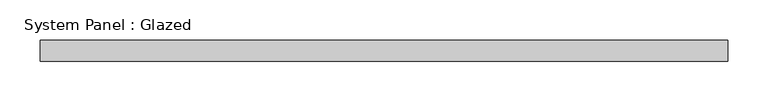
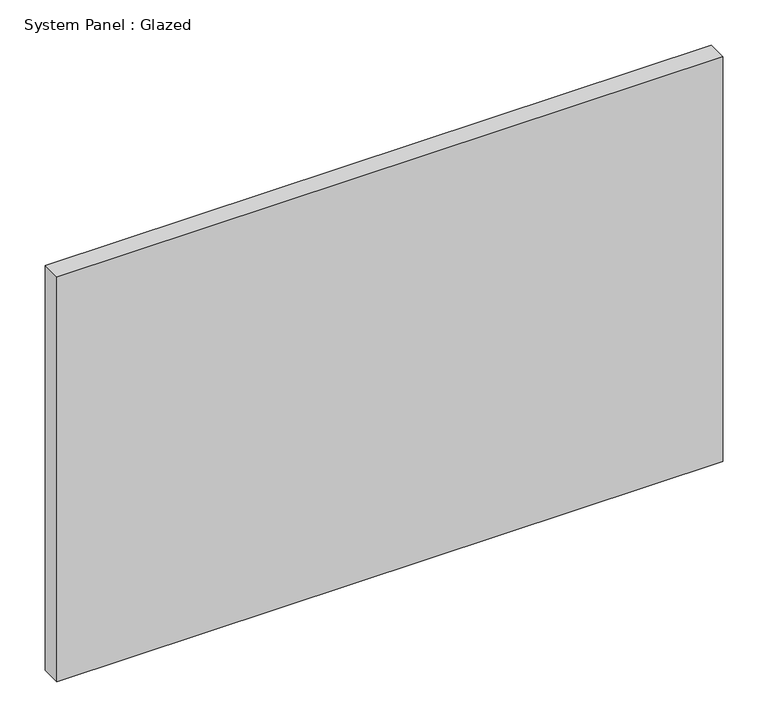
"""IFC4 building model written with IfcOpenShell, lengths in millimetres: plate geometry, System Panel : Glazed."""

from ifc_helpers import new_model, si_unit, origin, origin_with_axes, place, context, project, spatial, polyline, outline, extrude, source, transform, mapped, element, save


def system_panel_glazed_1cc9a2de(model_context):
    return source(origin(), model_context, "Body", "SweptSolid", [
        extrude(outline(polyline([(424.3916667, 19.05), (-424.3916667, 19.05), (-424.3916667, 44.45), (424.3916667, 44.45), (424.3916667, 19.05)])), origin_with_axes(), (0.0, 0.0, 1.0), 545.6538352),
    ])


if __name__ == "__main__":
    model = new_model("IFC4")
    model_context = context("Model", 3, world=origin())
    ifc_project = project(units=[si_unit("LENGTHUNIT", "METRE", prefix="MILLI")], contexts=[model_context])
    site = spatial("IfcSite", under=ifc_project)
    building = spatial("IfcBuilding", under=site)
    placement = place(None, origin())
    system_panel_glazed_shape = system_panel_glazed_1cc9a2de(model_context)
    element("IfcPlate", 1, ObjectType="System Panel : Glazed", at=placement, inside=building, context=model_context, shape_type="MappedRepresentation", body=[
        mapped(system_panel_glazed_shape, transform((0.0, 0.0, 0.0), x_axis=(1.0, 0.0, 0.0), y_axis=(0.0, 1.0, 0.0), z_axis=(0.0, 0.0, 1.0))),
    ])
    save(model, "model.ifc")

# Revit data of these elements
# Type "System Panel : Glazed"
#   Construction Type Id = "GSP4R"
#   Analytic Construction = "1/8 in Pilkington single glazing"
#   Visual Light Transmittance = 0.9
#   Solar Heat Gain Coefficient = 0.86
#   Heat Transfer Coefficient (U) = 1.18115 BTU/(h·ft²·°F)
#   Define Thermal Properties by = 1
# Element 1 (IfcPlate, "System Panel : Glazed")
#   Materials on its faces: "Glass"
# Materials
#   "Glass": class "Glass", colour RGB 0 128 192, transparency 0.75, Description = "Soda Lime Glass", Cost = 0
